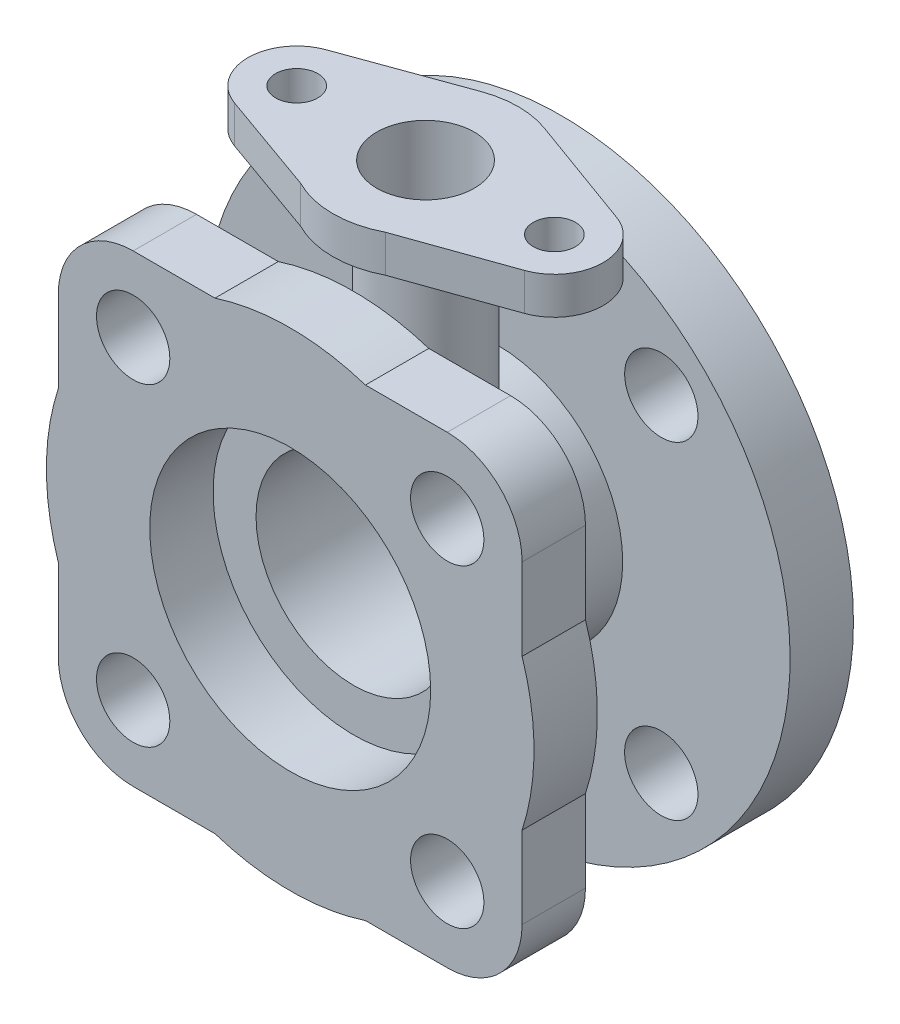
SolidWorks part; units mm, degrees
material "Plain Carbon Steel"
ref_plane "Front Plane" through (0, 0, 0) normal (0, 0, 1) x (1, 0, 0)
ref_plane "Top Plane" through (0, 0, 0) normal (0, 1, 0) x (1, 0, 0)
ref_plane "Right Plane" through (0, 0, 0) normal (1, 0, 0) x (0, 0, -1)
sketch "Round Flange Sketch" plane through (0, 0, 0) normal (0, 0, 1) x (1, 0, 0)
  circle A0 centre (0, 0) radius 76.2
  dimension "D1" = 152.4
extrude "Round Flange Ø152.4" add sketch "Round Flange Sketch" along normal blind 16.5
sketch "Hub Sketch" plane through (0, 0, 16.5) normal (0, 0, 1) x (1, 0, 0)
  circle A0 centre (0, 0) radius 32.6
  dimension "D1" = 65.2
extrude "Hub Ø65.2" add sketch "Hub Sketch" along normal blind 18.75
sketch "Tapered Neck Sketch" plane through (0, 0, 35.25) normal (0, 0, 1) x (1, 0, 0)
  circle A1 centre (0, 0) radius 32.6
  dimension "D1" = 65.2
extrude "Tapered Neck 12deg Draft" add sketch "Tapered Neck Sketch" along normal blind 18.75 draft 12 draft outward yes
sketch "Square Flange Sketch" plane through (0, 0, 54) normal (0, 0, 1) x (1, 0, 0)
  line L1 (19.5982, -60.4) -> (40.9, -60.4)
  line L7 (60.4, -40.9) -> (60.4, -19.5982)
  line L9 (-40.9, 60.4) -> (-19.5982, 60.4)
  line L10 (-60.4, 40.9) -> (-60.4, 19.5982)
  line L11 (-40.9, -60.4) -> (-19.5982, -60.4)
  line L12 (60.4, 19.5982) -> (60.4, 40.9)
  line L13 (19.5982, 60.4) -> (40.9, 60.4)
  line L14 (-60.4, -19.5982) -> (-60.4, -40.9)
  arc A7 (60.4, -19.5982) -> (60.4, 19.5982) centre (0, 0) ccw
  arc A9 (40.9, -60.4) -> (60.4, -40.9) centre (40.9, -40.9) ccw
  circle A10 centre (0, 0) radius 77.3413
  arc A11 (40.9, 60.4) -> (60.4, 40.9) centre (40.9, 40.9) cw
  arc A12 (-40.9, 60.4) -> (-60.4, 40.9) centre (-40.9, 40.9) ccw
  arc A13 (-40.9, -60.4) -> (-60.4, -40.9) centre (-40.9, -40.9) cw
  arc A14 (19.5982, 60.4) -> (-19.5982, 60.4) centre (0, 0) ccw
  arc A15 (-60.4, 19.5982) -> (-60.4, -19.5982) centre (0, 0) ccw
  arc A16 (-19.5982, -60.4) -> (19.5982, -60.4) centre (0, 0) ccw
  circle A17 centre (0, 0) radius 36.5854 construction
  circle M7 centre (0, 0) radius 36.5854
  dimension "D1" = 127
  dimension "D2" = 40.9
  dimension "D4" = 154.6827
  dimension "D5" = 19.5
  dimension "D6" = 19.5982
  dimension "D3" = 40.9
  dimension "D7" = 19.5982
extrude "Square Flange 127" add sketch "Square Flange Sketch" along normal blind 16.5 separate body contours L11 A16 L1 A9 L7 A7 L12 A11 L13 A14 L9 A12 L10 A15 L14 A13 M7
sketch "Square Flange Holes Sketch" plane through (0, 0, 70.5) normal (0, 0, 1) x (1, 0, 0)
  line L0 (0, 0) -> (26.6195, 0)
  line L1 (0, 0) -> (0, -15.3411)
  line L2 (60.4, -40.9) -> (60.4, -19.5982) construction
  line L3 (19.5982, -60.4) -> (40.9, -60.4) construction
  circle A0 centre (40.9, -40.9) radius 9.55
  circle A1 centre (40.9, 40.9) radius 9.55
  circle A2 centre (-40.9, -40.9) radius 9.55
  circle A3 centre (-40.9, 40.9) radius 9.55
  dimension "D1" = 19.1
  dimension "D2" = 33.7805
  dimension "D3" = 45.0589
extrude "Square Flange Holes" cut sketch "Square Flange Holes Sketch" against normal blind 20.5 contours A3 | A1 | A0 | A2
sketch "Round Flange Bolt Holes Sketch" plane through (0, 0, 0) normal (0, 0, -1) x (-1, 0, 0)
  circle A0 centre (42.65, -42.65) radius 9.55
  circle A1 centre (42.65, 42.65) radius 9.55
  circle A2 centre (-42.65, -42.65) radius 9.55
  circle A3 centre (-42.65, 42.65) radius 9.55
  dimension "D1" = 19.1
  dimension "D2" = 19.1
  dimension "D7" = 19.1
  dimension "D8" = 19.1
  dimension "D3" = 42.65
  dimension "D4" = 85.3
  dimension "D5" = 85.3
  dimension "D6" = 42.65
  dimension "D9" = 42.65
  dimension "D10" = 42.65
  dimension "D11" = 42.65
  dimension "D12" = 42.65
extrude "Round Flange Bolt Holes 4xØ19.1" cut sketch "Round Flange Bolt Holes Sketch" against normal blind 20.5
sketch "Square Flange Bore Sketch" plane through (0, 0, 70.5) normal (0, 0, 1) x (1, 0, 0)
  circle A0 centre (0, 0) radius 25.4
  dimension "D1" = 50.8
extrude "Square Flange Bore" cut sketch "Square Flange Bore Sketch" against normal blind 121
sketch "Side Port Boss Sketch" plane through (0, 0, 0) normal (0, 1, 0) x (1, 0, 0)
  line L0 (32.6, -35.25) -> (-32.6, -35.25) construction
  circle A0 centre (0, -35.25) radius 13.5
  dimension "D1" = 27
extrude "Side Port Boss" add sketch "Side Port Boss Sketch" along normal blind 74
sketch "Port Pad Sketch" plane through (0, 74, 0) normal (0, 1, 0) x (1, 0, 0)
  line L1 (-37.8843, -23.3125) -> (-8.242, -12.5499)
  line L2 (-37.8843, -47.1875) -> (-11.0096, -56.7444)
  line L3 (37.726, -47.2438) -> (11.0096, -56.7444)
  line L4 (37.8843, -23.3125) -> (8.242, -12.5499)
  arc A0 (8.242, -12.5499) -> (-8.242, -12.5499) centre (0, -35.25) ccw
  arc A1 (-37.8843, -23.3125) -> (-37.8843, -47.1875) centre (-33.55, -35.25) ccw
  arc A2 (37.8843, -23.3125) -> (37.726, -47.2438) centre (33.55, -35.25) cw
  arc A3 (-11.0096, -56.7444) -> (11.0096, -56.7444) centre (0, -35.25) ccw
  circle A4 centre (0, -35.25) radius 13.5 construction
  dimension "D1" = 24.15
  dimension "D2" = 12.7
  dimension "D3" = 8.242
  dimension "D4" = 11.0096
  dimension "D6" = 37.726
extrude "Port Pad" add sketch "Port Pad Sketch" along normal blind 9.7
sketch "Round Flange Bore Sketch" plane through (0, 0, 54) normal (0, 0, 1) x (1, 0, 0)
  circle A0 centre (0, 0) radius 25.4
  dimension "D1" = 50.8
extrude "Round Flange Bore" cut sketch "Round Flange Bore Sketch" against normal blind 352.7
sketch "Pad Bolt Holes Sketch" plane through (0, 83.7, 0) normal (0, 1, 0) x (1, 0, 0)
  circle A0 centre (33.55, -35.25) radius 5.5
  circle A1 centre (-33.55, -35.25) radius 5.5
  dimension "D1" = 11
extrude "Pad Bolt Holes 2x" cut sketch "Pad Bolt Holes Sketch" against normal blind 32.7
sketch "Side Port Bore Sketch" plane through (0, 83.7, 0) normal (0, 1, 0) x (1, 0, 0)
  circle A0 centre (0, -35.25) radius 12.7
  dimension "D1" = 25.4
extrude "Side Port Bore" cut sketch "Side Port Bore Sketch" against normal blind 74.7
